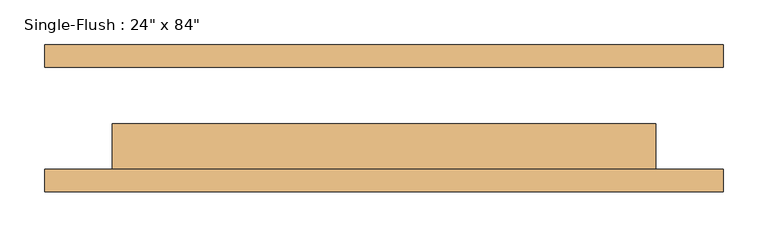
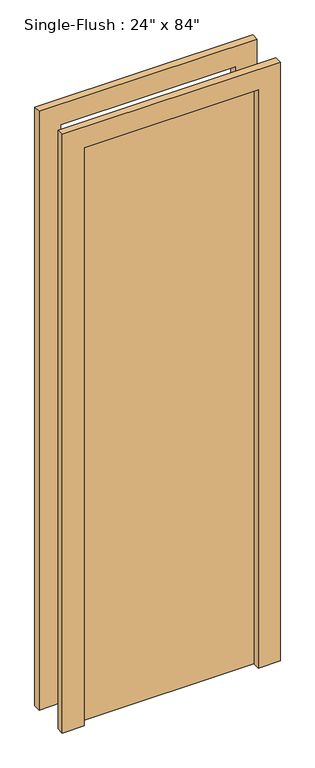
"""IFC4 building model written with IfcOpenShell, lengths in millimetres: door geometry."""

from ifc_helpers import new_model, si_unit, frame, origin, origin_with_axes, place, context, project, spatial, polyline, outline, extrude, source, transform, mapped, element, save


def door_0bf9f8da(model_context):
    return source(origin(), model_context, "Body", "SweptSolid", [
        extrude(outline(polyline([(2209.8, -381.0), (0.0, -381.0), (0.0, -304.8), (2133.6, -304.8), (2133.6, 304.8), (0.0, 304.8), (0.0, 381.0), (2209.8, 381.0), (2209.8, -381.0)])), frame((0.0, -82.55, 0.0), z_axis=(0.0, 1.0, 0.0), x_axis=(0.0, 0.0, 1.0)), (0.0, 0.0, 1.0), 25.4),
        extrude(outline(polyline([(2209.8, 381.0), (2209.8, -381.0), (0.0, -381.0), (0.0, -304.8), (2133.6, -304.8), (2133.6, 304.8), (0.0, 304.8), (0.0, 381.0), (2209.8, 381.0)])), frame((0.0, 57.15, 0.0), z_axis=(0.0, 1.0, 0.0), x_axis=(0.0, 0.0, 1.0)), (0.0, 0.0, 1.0), 25.4),
        extrude(outline(polyline([(304.8, -6.35), (304.8, -57.15), (-304.8, -57.15), (-304.8, -6.35), (304.8, -6.35)])), origin_with_axes(), (0.0, 0.0, 1.0), 2133.6),
    ])


if __name__ == "__main__":
    model = new_model("IFC4")
    model_context = context("Model", 3, world=origin())
    ifc_project = project(units=[si_unit("LENGTHUNIT", "METRE", prefix="MILLI")], contexts=[model_context])
    site = spatial("IfcSite", under=ifc_project)
    building = spatial("IfcBuilding", under=site)
    placement = place(None, origin())
    door_shape = door_0bf9f8da(model_context)
    element("IfcDoor", 1, ObjectType="Single-Flush : 24\" x 84\"", at=placement, inside=building, context=model_context, shape_type="MappedRepresentation", body=[
        mapped(door_shape, transform((0.0, 0.0, 0.0), x_axis=(1.0, 0.0, 0.0), y_axis=(0.0, 1.0, 0.0), z_axis=(0.0, 0.0, 1.0))),
    ])
    save(model, "model.ifc")

# Revit data of these elements
# Type "Single-Flush : 24\" x 84\""
#   Type Mark = "1"
#   Construction Type Id = "MDOOR"
#   Assembly Code = "C1020"
#   Analytic Construction = "Metal"
#   Thickness = 0' - 2"
#   Heat Transfer Coefficient (U) = 0.651978 BTU/(h·ft²·°F)
#   Height = 7' - 0"
#   Trim Projection Ext = 0' - 1"
#   Trim Projection Int = 0' - 1"
#   Trim Width = 0' - 3"
#   Width = 2' - 0"
#   Define Thermal Properties by = 1
#   Define Thermal Properties by = 1
#   Door Material = Door - Panel
#   Frame Material = Door - Frame
#   Visual Light Transmittance = 0
#   Solar Heat Gain Coefficient = 0
#   Function = (empty or 0)
#   Wall Closure = (empty or 0)
# Element 1 (IfcDoor, "Single-Flush : 24\" x 84\"")
#   Materials on its faces: "Door - Frame", "Door - Panel"
# Materials
#   "Door - Panel": class "Wood", colour RGB 210 159 95, transparency 0, Cost = 0
#   "Door - Frame": colour RGB 118 70 51, transparency 0, Cost = 0
